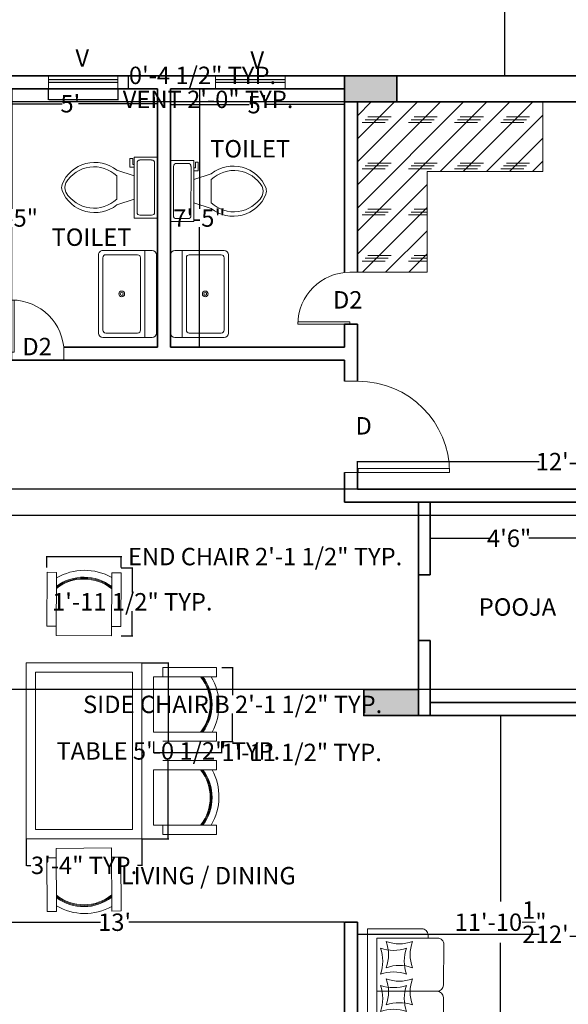
# Model space of a CAD drawing. Units: inches. Extents: x -2181 to 1225, y -80 to 4016.
# Tile 3 of 10: x 308 to 497, y 253 to 592. Entities that reach past the tile are written whole.
import ezdxf

# ---------------------------------------------------------------- set-up
doc = ezdxf.new("R2010")
doc.units = ezdxf.units.IN
doc.header["$MEASUREMENT"] = 0
for name, color, linetype, lineweight in [('A-ANNO-DIMS', 2, 'Continuous', 18), ('A-ANNO-TEXT', 7, 'Continuous', 18), ('A-AREA-IDEN', 7, 'Continuous', 18), ('A-COLS', 7, 'Continuous', 35), ('A-COLS-PATT', 252, 'Continuous', 13), ('A-DOOR', 3, 'Continuous', 18), ('A-FLOR-FIXT', 8, 'Continuous', 18), ('A-FURN', 30, 'Continuous', 18), ('A-GLAZ', 4, 'Continuous', 18), ('A-GLAZ-PATT', 4, 'Continuous', 13), ('A-MILL', 8, 'Continuous', 18), ('A-MILL-PATT', 252, 'Continuous', 13), ('A-WALL', 7, 'Continuous', 35)]:
    doc.layers.add(name, color=color, linetype=linetype, lineweight=lineweight)
doc.styles.get("Standard").update_dxf_attribs({"font": 'arial.ttf'})
doc.dimstyles.get("Standard").update_dxf_attribs({"dimtxt": 6, "dimasz": 0.18, "dimexe": 0.18, "dimexo": 0.0625, "dimgap": 0.09, "dimtad": 0, "dimtih": 1, "dimtoh": 1, "dimdec": 4, "dimzin": 0, "dimdsep": 46, "dimlunit": 4, "dimtxsty": 'Standard', "dimcen": 0.09, "dimadec": 0, "dimazin": 0, "dimtfac": 1, "dimtdec": 4, "dimtofl": 0, "dimtmove": 0, "dimatfit": 3, "dimfxl": 1, "dimtolj": 1, "dimtzin": 0, "dimarcsym": 0})

# ---------------------------------------------------------------- blocks, each defined once
blk = doc.blocks.new('*U2')
for p, q in [((0, 0), (0, -6)), ((40, 0), (40, -6))]:
    blk.add_line(p, q)
blk.add_lwpolyline([(0, 0), (0, 40), (1.75, 40), (1.75, 0)], close=True)
blk.add_arc((0, 0), 40, 0, 90)
blk = doc.blocks.new('*U21')
for p, q in [((9.5, -6), (9.5, -2)), ((-10, -8.5), (-8, -8.5)), ((-10, -9.5), (-10, -8.5)), ((-7, -9.5), (-10, -9.5)), ((-8, -8.5), (-8, -8)), ((-7, -8), (-7, -9.5)), ((-4, -8), (-6, -14)), ((4, -8), (6, -14)), ((4, -14), (-4, -14))]:
    blk.add_line(p, q)
blk.add_lwpolyline([(10.5, -8), (10.5, 0), (-10.5, 0), (-10.5, -8)], close=True)
for points in [[(-9.5, -2), (-9.5, -6)], [(8.5, -1), (-8.5, -1)], [(-8.5, -7), (8.5, -7)]]:
    blk.add_lwpolyline(points)
for centre, radius, start, end in [((-8.62, -1.88), 0.884, 81.8699, 188.1301), ((8.62, -1.88), 0.884, 351.8699, 98.1301), ((-8.62, -6.12), 0.884, 171.8699, 278.1301), ((8.62, -6.12), 0.884, 261.8699, 8.1301), ((3.52, -21.58), 12.17, 141.4691, 247.9714), ((4.2, -21.82), 11.33, 136.3677, 238.9468), ((-3.52, -21.58), 12.17, 292.0284, 38.5307), ((-4.2, -21.82), 11.33, 301.053, 43.6321), ((0, -27.88), 4, 245.7318, 294.2682), ((0, -29), 4, 254.8605, 285.1395)]:
    blk.add_arc(centre, radius, start, end)
blk = doc.blocks.new('Sink-single - 30 in top')
blk.add_line((-15, -3.999996), (15, -3.999996))
for points in [[(-13.5, 0), (13.5, 0)], [(-15, -18.499996), (-15, -1.5)], [(15, -1.5), (15, -18.499996)], [(-13.5, -17.499996), (-13.5, -6.499996)], [(-12.5, -5.499996), (12.5, -5.499996)], [(13.5, -6.499996), (13.5, -17.499996)], [(13.5, -19.999996), (-13.5, -19.999996)], [(12.5, -18.499996), (-12.5, -18.499996)]]:
    blk.add_lwpolyline(points)
for radius in [1, 0.5]:
    blk.add_circle((0, -11.999996), radius)
for centre, radius, start, end in [((-13.5, -1.5), 1.5, 90, 180), ((13.5, -1.5), 1.5, 0, 90), ((-12.5, -6.499996), 1, 90, 180), ((12.5, -6.499996), 1, 0, 90), ((-13.5, -18.499996), 1.5, 180, 270), ((-12.5, -17.499996), 1, 180, 270), ((12.5, -17.499996), 1, 270, 0), ((13.5, -18.499996), 1.5, 270, 0)]:
    blk.add_arc(centre, radius, start, end)
blk = doc.blocks.new('*D22')
at = {"layer": 'A-ANNO-DIMS', "color": 0, "lineweight": -2, "transparency": 16777216}
for p, q in [((470.02, 664.48), (474.9, 664.48)), ((474.72, 664.3), (474.72, 625.85)), ((474.72, 573.16), (474.72, 611.62)), ((624.01, 572.98), (474.54, 572.98))]:
    blk.add_line(p, q, dxfattribs=at)
at = {"layer": 'A-ANNO-DIMS', "color": 0, "transparency": 16777216}
for points in [[(474.69, 664.3), (474.75, 664.3), (474.72, 664.48)], [(474.69, 573.16), (474.75, 573.16), (474.72, 572.98)]]:
    blk.add_solid(points, dxfattribs=at)
at = {"layer": 'Defpoints', "color": 0, "transparency": 16777216}
for p in [(469.95, 664.48), (474.72, 572.98), (624.08, 572.98)]:
    blk.add_point(p, dxfattribs=at)
at = {"layer": 'A-ANNO-DIMS', "color": 0, "transparency": 16777216, "insert": (474.72, 618.73), "char_height": 6, "attachment_point": 5}
blk.add_mtext('\\A1;7\'-7{\\H1x;\\S1/2;}"', dxfattribs=at)
blk = doc.blocks.new('*D26')
at = {"layer": 'A-ANNO-DIMS', "color": 0, "lineweight": -2, "transparency": 16777216}
for p, q in [((295.08, 568.48), (305, 568.48)), ((304.82, 568.3), (304.82, 527.13)), ((304.82, 479.66), (304.82, 520.84)), ((295.08, 479.48), (305, 479.48))]:
    blk.add_line(p, q, dxfattribs=at)
at = {"layer": 'A-ANNO-DIMS', "color": 0, "transparency": 16777216}
for points in [[(304.79, 568.3), (304.85, 568.3), (304.82, 568.48)], [(304.79, 479.66), (304.85, 479.66), (304.82, 479.48)]]:
    blk.add_solid(points, dxfattribs=at)
at = {"layer": 'Defpoints', "color": 0, "transparency": 16777216}
for p in [(295.01, 568.48), (295.01, 479.48), (304.82, 479.48)]:
    blk.add_point(p, dxfattribs=at)
at = {"layer": 'A-ANNO-DIMS', "color": 0, "transparency": 16777216, "insert": (304.82, 523.98), "char_height": 6, "attachment_point": 5}
blk.add_mtext('\\A1;7\'-5"', dxfattribs=at)
blk = doc.blocks.new('*D27')
at = {"layer": 'A-ANNO-DIMS', "color": 0, "lineweight": -2, "transparency": 16777216}
for p, q in [((359.58, 568.48), (369.69, 568.48)), ((369.51, 568.3), (369.51, 527.13)), ((369.51, 479.66), (369.51, 520.84)), ((359.58, 479.48), (369.69, 479.48))]:
    blk.add_line(p, q, dxfattribs=at)
at = {"layer": 'A-ANNO-DIMS', "color": 0, "transparency": 16777216}
for points in [[(369.48, 568.3), (369.54, 568.3), (369.51, 568.48)], [(369.48, 479.66), (369.54, 479.66), (369.51, 479.48)]]:
    blk.add_solid(points, dxfattribs=at)
at = {"layer": 'Defpoints', "color": 0, "transparency": 16777216}
for p in [(359.51, 568.48), (359.51, 479.48), (369.51, 479.48)]:
    blk.add_point(p, dxfattribs=at)
at = {"layer": 'A-ANNO-DIMS', "color": 0, "transparency": 16777216, "insert": (369.51, 523.98), "char_height": 6, "attachment_point": 5}
blk.add_mtext('\\A1;7\'-5"', dxfattribs=at)
blk = doc.blocks.new('*D28')
at = {"layer": 'A-ANNO-DIMS', "color": 0, "lineweight": -2, "transparency": 16777216}
for p, q in [((295.01, 568.42), (295.01, 563.2)), ((355.01, 568.42), (355.01, 563.2)), ((295.19, 563.38), (322.16, 563.38)), ((354.83, 563.38), (327.87, 563.38))]:
    blk.add_line(p, q, dxfattribs=at)
at = {"layer": 'A-ANNO-DIMS', "color": 0, "transparency": 16777216}
for points in [[(295.19, 563.41), (295.19, 563.35), (295.01, 563.38)], [(354.83, 563.41), (354.83, 563.35), (355.01, 563.38)]]:
    blk.add_solid(points, dxfattribs=at)
at = {"layer": 'Defpoints', "color": 0, "transparency": 16777216}
for p in [(295.01, 568.48), (355.01, 568.48), (355.01, 563.38)]:
    blk.add_point(p, dxfattribs=at)
at = {"layer": 'A-ANNO-DIMS', "color": 0, "transparency": 16777216, "insert": (325.01, 563.38), "char_height": 6, "attachment_point": 5}
blk.add_mtext("\\A1;5'", dxfattribs=at)
blk = doc.blocks.new('*D29')
at = {"layer": 'A-ANNO-DIMS', "color": 0, "lineweight": -2, "transparency": 16777216}
for p, q in [((359.51, 568.42), (359.51, 562.88)), ((419.51, 568.42), (419.51, 562.88)), ((359.69, 563.06), (386.66, 563.06)), ((419.33, 563.06), (392.37, 563.06))]:
    blk.add_line(p, q, dxfattribs=at)
at = {"layer": 'A-ANNO-DIMS', "color": 0, "transparency": 16777216}
for points in [[(359.69, 563.09), (359.69, 563.03), (359.51, 563.06)], [(419.33, 563.09), (419.33, 563.03), (419.51, 563.06)]]:
    blk.add_solid(points, dxfattribs=at)
at = {"layer": 'Defpoints', "color": 0, "transparency": 16777216}
for p in [(359.51, 568.48), (419.51, 568.48), (419.51, 563.06)]:
    blk.add_point(p, dxfattribs=at)
at = {"layer": 'A-ANNO-DIMS', "color": 0, "transparency": 16777216, "insert": (389.51, 563.06), "char_height": 6, "attachment_point": 5}
blk.add_mtext("\\A1;5'", dxfattribs=at)
blk = doc.blocks.new('*D43')
at = {"layer": 'A-ANNO-DIMS', "color": 0, "lineweight": -2, "transparency": 16777216}
for p, q in [((424.01, 281.17), (424.01, 276.89)), ((424.19, 277.07), (486.63, 277.07)), ((578.33, 277.07), (515.9, 277.07)), ((578.51, 277.13), (578.51, 277.25))]:
    blk.add_line(p, q, dxfattribs=at)
at = {"layer": 'A-ANNO-DIMS', "color": 0, "transparency": 16777216}
for points in [[(424.19, 277.1), (424.19, 277.04), (424.01, 277.07)], [(578.33, 277.1), (578.33, 277.04), (578.51, 277.07)]]:
    blk.add_solid(points, dxfattribs=at)
at = {"layer": 'Defpoints', "color": 0, "transparency": 16777216}
for p in [(424.01, 281.23), (578.51, 277.07), (578.51, 277.07)]:
    blk.add_point(p, dxfattribs=at)
at = {"layer": 'A-ANNO-DIMS', "color": 0, "transparency": 16777216, "insert": (501.26, 277.07), "char_height": 6, "attachment_point": 5}
blk.add_mtext('\\A1;12\'-10{\\H1x;\\S1/2;}"', dxfattribs=at)
blk = doc.blocks.new('*D44')
at = {"layer": 'A-ANNO-DIMS', "color": 0, "lineweight": -2, "transparency": 16777216}
for p, q in [((473.3, 352.3), (473.3, 288.4)), ((473.37, 352.48), (473.48, 352.48)), ((473.3, 210.16), (473.3, 274.07)), ((473.37, 209.98), (473.48, 209.98))]:
    blk.add_line(p, q, dxfattribs=at)
at = {"layer": 'A-ANNO-DIMS', "color": 0, "transparency": 16777216}
for points in [[(473.27, 352.3), (473.33, 352.3), (473.3, 352.48)], [(473.27, 210.16), (473.33, 210.16), (473.3, 209.98)]]:
    blk.add_solid(points, dxfattribs=at)
at = {"layer": 'Defpoints', "color": 0, "transparency": 16777216}
for p in [(473.3, 352.48), (473.3, 352.48), (473.3, 209.98)]:
    blk.add_point(p, dxfattribs=at)
at = {"layer": 'A-ANNO-DIMS', "color": 0, "transparency": 16777216, "insert": (473.3, 281.23), "char_height": 6, "attachment_point": 5}
blk.add_mtext('\\A1;11\'-10{\\H1x;\\S1/2;}"', dxfattribs=at)
blk = doc.blocks.new('*D45')
at = {"layer": 'A-ANNO-DIMS', "color": 0, "lineweight": -2, "transparency": 16777216}
for p, q in [((449.01, 425.92), (449.01, 413.4)), ((503.46, 425.92), (503.46, 413.4)), ((449.19, 413.58), (469.45, 413.58)), ((503.28, 413.58), (483.03, 413.58))]:
    blk.add_line(p, q, dxfattribs=at)
at = {"layer": 'A-ANNO-DIMS', "color": 0, "transparency": 16777216}
for points in [[(449.19, 413.61), (449.19, 413.55), (449.01, 413.58)], [(503.28, 413.61), (503.28, 413.55), (503.46, 413.58)]]:
    blk.add_solid(points, dxfattribs=at)
at = {"layer": 'Defpoints', "color": 0, "transparency": 16777216}
for p in [(449.01, 425.98), (503.46, 425.98), (503.46, 413.58)]:
    blk.add_point(p, dxfattribs=at)
at = {"layer": 'A-ANNO-DIMS', "color": 0, "transparency": 16777216, "insert": (476.24, 413.58), "char_height": 6, "width": 24.618, "attachment_point": 5}
blk.add_mtext('\\A1;4\'6"', dxfattribs=at)
blk = doc.blocks.new('*D48')
at = {"layer": 'A-ANNO-DIMS', "color": 0, "lineweight": -2, "transparency": 16777216}
for p, q in [((424.01, 430.55), (424.01, 440.19)), ((424.19, 440.01), (486.63, 440.01)), ((578.33, 440.01), (515.9, 440.01)), ((578.51, 430.55), (578.51, 440.19))]:
    blk.add_line(p, q, dxfattribs=at)
at = {"layer": 'A-ANNO-DIMS', "color": 0, "transparency": 16777216}
for points in [[(424.19, 440.04), (424.19, 439.98), (424.01, 440.01)], [(578.33, 440.04), (578.33, 439.98), (578.51, 440.01)]]:
    blk.add_solid(points, dxfattribs=at)
at = {"layer": 'Defpoints', "color": 0, "transparency": 16777216}
for p in [(578.51, 440.01), (424.01, 430.48), (578.51, 430.48)]:
    blk.add_point(p, dxfattribs=at)
at = {"layer": 'A-ANNO-DIMS', "color": 0, "transparency": 16777216, "insert": (501.26, 440.01), "char_height": 6, "attachment_point": 5}
blk.add_mtext('\\A1;12\'-10{\\H1x;\\S1/2;}"', dxfattribs=at)
blk = doc.blocks.new('*D49')
at = {"layer": 'A-ANNO-DIMS', "color": 0, "lineweight": -2, "transparency": 16777216}
for p, q in [((261.01, 284.15), (261.01, 281.05)), ((261.19, 281.23), (335.37, 281.23)), ((419.33, 281.23), (345.16, 281.23)), ((419.51, 281.3), (419.51, 281.41))]:
    blk.add_line(p, q, dxfattribs=at)
at = {"layer": 'A-ANNO-DIMS', "color": 0, "transparency": 16777216}
for points in [[(261.19, 281.26), (261.19, 281.2), (261.01, 281.23)], [(419.33, 281.26), (419.33, 281.2), (419.51, 281.23)]]:
    blk.add_solid(points, dxfattribs=at)
at = {"layer": 'Defpoints', "color": 0, "transparency": 16777216}
for p in [(261.01, 284.21), (419.51, 281.23), (419.51, 281.23)]:
    blk.add_point(p, dxfattribs=at)
at = {"layer": 'A-ANNO-DIMS', "color": 0, "transparency": 16777216, "insert": (340.26, 281.23), "char_height": 6, "attachment_point": 5}
blk.add_mtext("\\A1;13'", dxfattribs=at)
blk = doc.blocks.new('*D71')
at = {"layer": 'A-ANNO-DIMS', "color": 0, "lineweight": -2, "transparency": 16777216}
for p, q in [((98.51, 573.05), (98.51, 611.58)), ((98.69, 611.4), (536.64, 611.4)), ((995.33, 611.4), (557.39, 611.4)), ((995.51, 573.05), (995.51, 611.58))]:
    blk.add_line(p, q, dxfattribs=at)
at = {"layer": 'A-ANNO-DIMS', "color": 0, "transparency": 16777216}
for points in [[(98.69, 611.43), (98.69, 611.37), (98.51, 611.4)], [(995.33, 611.43), (995.33, 611.37), (995.51, 611.4)]]:
    blk.add_solid(points, dxfattribs=at)
at = {"layer": 'Defpoints', "color": 0, "transparency": 16777216}
for p in [(995.51, 611.4), (98.51, 572.98), (995.51, 572.98)]:
    blk.add_point(p, dxfattribs=at)
at = {"layer": 'A-ANNO-DIMS', "color": 0, "transparency": 16777216, "insert": (547.01, 611.4), "char_height": 6, "attachment_point": 5}
blk.add_mtext('\\A1;74\'-9"', dxfattribs=at)
blk = doc.blocks.new('SOFA-UPHOLSTERED')
for p, q in [((3.23, 44.91), (24.04, 44.91)), ((3.23, 22.57), (24.04, 22.58)), ((25.11, 22.58), (25.11, 22.58))]:
    blk.add_line(p, q)
for points in [[(0, 0), (0, 66.42), (18.76, 66.42, -0.414214), (20.91, 64.27), (20.91, 63.19)], [(3.23, 3.23), (3.23, 63.19), (24.21, 63.19, -0.417877), (26.36, 61.02), (26.19, 47.04, -0.410559), (24.04, 44.91), (3.23, 44.91)], [(26.19, 42.76), (26.19, 24.73, -0.414214), (24.04, 22.58), (3.23, 22.58)], [(26.19, 20.43), (26.19, 5.38, -0.414214), (24.04, 3.23), (3.23, 3.23)], [(21.99, 3.23), (21.99, 3.23, -0.414214), (18.76, 0), (0, 0)]]:
    blk.add_lwpolyline(points, format="xyb")
for points in [[(18.76, 66.42), (19, 66.42)], [(19, 0), (18.76, 0)]]:
    blk.add_lwpolyline(points)
for centre, radius, start, end in [((11.03, 74.56), 13.33, 250.2663, 289.7337), ((-6.02, 57.51), 13.33, 340.2663, 19.7337), ((28.07, 57.51), 13.33, 160.2663, 199.7337), ((9.03, 72.31), 13.33, 250.2663, 289.7337), ((-8.02, 55.27), 13.33, 340.2663, 19.7337), ((26.07, 55.27), 13.33, 160.2663, 199.7337), ((9.03, 38.22), 13.33, 70.2663, 109.7337), ((11.03, 40.47), 13.33, 70.2663, 109.7337), ((11.03, 61.71), 13.33, 250.2663, 289.7337), ((-6.02, 44.66), 13.33, 340.2663, 19.7337), ((28.07, 44.66), 13.33, 160.2663, 199.7337), ((9.03, 59.47), 13.33, 250.2663, 289.7337), ((-8.02, 42.42), 13.33, 340.2663, 19.7337), ((26.07, 42.42), 13.33, 160.2663, 199.7337), ((24.04, 42.76), 2.15, 360, 90), ((11.03, 27.62), 13.33, 70.2663, 109.7337), ((9.03, 25.38), 13.33, 70.2663, 109.7337), ((11.72, 48.03), 13.33, 250.2663, 289.7337), ((-5.33, 30.99), 13.33, 340.2663, 19.7337), ((28.76, 30.99), 13.33, 160.2663, 199.7337), ((9.72, 45.79), 13.33, 250.2663, 289.7337), ((-7.33, 28.74), 13.33, 340.2663, 19.7337), ((26.76, 28.74), 13.33, 160.2663, 199.7337), ((11.72, 13.94), 13.33, 70.2663, 109.7337), ((9.72, 11.7), 13.33, 70.2663, 109.7337), ((24.04, 20.43), 2.15, 0, 90.0249), ((9.86, 27), 13.33, 250.2663, 289.7337), ((-7.19, 9.96), 13.33, 340.2663, 19.7337), ((11.86, 29.25), 13.33, 250.2663, 289.7337), ((-5.19, 12.2), 13.33, 340.2663, 19.7337), ((26.9, 9.96), 13.33, 160.2663, 199.7337), ((28.9, 12.2), 13.33, 160.2663, 199.7337), ((11.86, -4.84), 13.33, 70.2663, 109.7337), ((9.86, -7.09), 13.33, 70.2663, 109.7337)]:
    blk.add_arc(centre, radius, start, end)
blk = doc.blocks.new('DINING-CHAIR-SIDE-B')
for p, q in [((3.21, 22.26), (3.21, 25.47)), ((21.75, 22.26), (21.75, 25.47)), ((21.75, 0), (21.75, 3.21))]:
    blk.add_line(p, q)
for points in [[(21.75, 25.47), (3.21, 25.47)], [(21.75, 22.26), (0, 22.26), (0, 3.21), (21.75, 3.21)], [(3.21, 0), (21.75, 0)]]:
    blk.add_lwpolyline(points)
for centre, radius, start, end in [((4.25, 12.73), 15.28, 321.4242, 38.5758), ((4.25, 12.73), 15.6, 322.3578, 37.6422), ((4.25, 12.73), 15.92, 323.2428, 36.7572), ((3.41, 12.45), 19.13, 331.1027, 30.8582)]:
    blk.add_arc(centre, radius, start, end)
blk = doc.blocks.new('DINING-CHAIR-END')
for p, q in [((3.21, 19.25), (0, 19.23)), ((22.26, 19.4), (25.47, 19.42)), ((25.38, 19.42), (25.38, 19.34)), ((3.35, 0.72), (0.14, 0.69)), ((25.61, 0.89), (22.4, 0.86))]:
    blk.add_line(p, q)
for points in [[(3.35, 0.72), (3.18, 22.46), (22.23, 22.61), (22.4, 0.86)], [(0.14, 0.69), (0, 19.23)], [(25.47, 19.42), (25.61, 0.89)]]:
    blk.add_lwpolyline(points)
for centre, radius, start, end in [((12.74, 18.29), 15.28, 231.8612, 309.0129), ((12.74, 18.29), 15.6, 232.7948, 308.0793), ((12.74, 18.29), 15.92, 233.6799, 307.1942), ((13.02, 19.13), 19.13, 239.5789, 299.3344)]:
    blk.add_arc(centre, radius, start, end)
blk = doc.blocks.new('DINING-TABLE')
for points in [[(39.83, 60.67), (39.83, 0), (0, 0), (0, 60.67)], [(36.62, 57.46), (36.62, 3.21), (3.21, 3.21), (3.21, 57.46)]]:
    blk.add_lwpolyline(points, close=True)
blk = doc.blocks.new('COL-18X9')
blk.add_lwpolyline([(0, 9), (18, 9), (18, 0), (0, 0)], close=True)
blk = doc.blocks.new('COL-18.89X9')
blk.add_lwpolyline([(18.9, 9), (0, 9), (0, 0), (18.9, 0)], close=True)
blk = doc.blocks.new('VENT-24')
for p, q in [((0, 0), (0, 4.5)), ((24, 0), (24, 4.5)), ((0, 3.25), (24, 3.25)), ((0, 2.25), (24, 2.25))]:
    blk.add_line(p, q)
blk = doc.blocks.new('*D100')
at = {"layer": 'A-ANNO-DIMS', "color": 0, "lineweight": -2, "transparency": 16777216}
for p, q in [((316.92, 403.49), (316.92, 407.45)), ((342.53, 403.49), (342.53, 407.45)), ((317.1, 407.27), (342.35, 407.27)), ((342.53, 407.27), (342.71, 407.27))]:
    blk.add_line(p, q, dxfattribs=at)
at = {"layer": 'A-ANNO-DIMS', "color": 0, "transparency": 16777216}
for points in [[(317.1, 407.3), (317.1, 407.24), (316.92, 407.27)], [(342.35, 407.3), (342.35, 407.24), (342.53, 407.27)]]:
    blk.add_solid(points, dxfattribs=at)
at = {"layer": 'Defpoints', "color": 0, "transparency": 16777216}
for p in [(342.53, 407.27), (316.92, 403.43), (342.53, 403.43)]:
    blk.add_point(p, dxfattribs=at)
at = {"layer": 'A-ANNO-DIMS', "color": 0, "transparency": 16777216, "insert": (392.14, 407.27), "char_height": 6, "attachment_point": 5}
blk.add_mtext('\\A1;END CHAIR 2\'-1 1/2" TYP.', dxfattribs=at)
blk = doc.blocks.new('*D101')
at = {"layer": 'A-ANNO-DIMS', "color": 0, "lineweight": -2, "transparency": 16777216}
for p, q in [((342.59, 403.43), (346.55, 403.43)), ((346.37, 403.25), (346.37, 394.87)), ((346.37, 380.12), (346.37, 388.49)), ((342.59, 379.94), (346.55, 379.94))]:
    blk.add_line(p, q, dxfattribs=at)
at = {"layer": 'A-ANNO-DIMS', "color": 0, "transparency": 16777216}
for points in [[(346.34, 403.25), (346.4, 403.25), (346.37, 403.43)], [(346.34, 380.12), (346.4, 380.12), (346.37, 379.94)]]:
    blk.add_solid(points, dxfattribs=at)
at = {"layer": 'Defpoints', "color": 0, "transparency": 16777216}
for p in [(342.53, 403.43), (342.53, 379.94), (346.37, 379.94)]:
    blk.add_point(p, dxfattribs=at)
at = {"layer": 'A-ANNO-DIMS', "color": 0, "transparency": 16777216, "insert": (346.37, 391.68), "char_height": 6, "attachment_point": 5}
blk.add_mtext('\\A1;1\'-11 1/2" TYP.', dxfattribs=at)
blk = doc.blocks.new('*D108')
at = {"layer": 'A-ANNO-DIMS', "color": 0, "lineweight": -2, "transparency": 16777216}
for p, q in [((377.2, 369.05), (381.14, 369.05)), ((380.96, 368.87), (380.96, 359.51)), ((380.96, 343.76), (380.96, 353.12)), ((377.2, 343.58), (381.14, 343.58))]:
    blk.add_line(p, q, dxfattribs=at)
at = {"layer": 'A-ANNO-DIMS', "color": 0, "transparency": 16777216}
for points in [[(380.93, 368.87), (380.99, 368.87), (380.96, 369.05)], [(380.93, 343.76), (380.99, 343.76), (380.96, 343.58)]]:
    blk.add_solid(points, dxfattribs=at)
at = {"layer": 'Defpoints', "color": 0, "transparency": 16777216}
for p in [(377.14, 369.05), (380.96, 369.05), (377.14, 343.58)]:
    blk.add_point(p, dxfattribs=at)
at = {"layer": 'A-ANNO-DIMS', "color": 0, "transparency": 16777216, "insert": (380.96, 356.32), "char_height": 6, "attachment_point": 5}
blk.add_mtext('\\A1;SIDE CHAIR B 2\'-1 1/2" TYP.', dxfattribs=at)
blk = doc.blocks.new('*D109')
at = {"layer": 'A-ANNO-DIMS', "color": 0, "lineweight": -2, "transparency": 16777216}
for p, q in [((353.7, 343.52), (353.7, 339.58)), ((377.14, 343.52), (377.14, 339.58)), ((353.88, 339.76), (376.96, 339.76)), ((377.14, 339.76), (377.32, 339.76))]:
    blk.add_line(p, q, dxfattribs=at)
at = {"layer": 'A-ANNO-DIMS', "color": 0, "transparency": 16777216}
for points in [[(353.88, 339.79), (353.88, 339.73), (353.7, 339.76)], [(376.96, 339.79), (376.96, 339.73), (377.14, 339.76)]]:
    blk.add_solid(points, dxfattribs=at)
at = {"layer": 'Defpoints', "color": 0, "transparency": 16777216}
for p in [(353.7, 343.58), (377.14, 343.58), (377.14, 339.76)]:
    blk.add_point(p, dxfattribs=at)
at = {"layer": 'A-ANNO-DIMS', "color": 0, "transparency": 16777216, "insert": (404.73, 339.76), "char_height": 6, "attachment_point": 5}
blk.add_mtext('\\A1;1\'-11 1/2" TYP.', dxfattribs=at)
blk = doc.blocks.new('*D110')
at = {"layer": 'A-ANNO-DIMS', "color": 0, "lineweight": -2, "transparency": 16777216}
for p, q in [((349.74, 370.6), (358.96, 370.6)), ((358.78, 370.42), (358.78, 343.46)), ((358.78, 310.11), (358.78, 337.07)), ((349.74, 309.93), (358.96, 309.93))]:
    blk.add_line(p, q, dxfattribs=at)
at = {"layer": 'A-ANNO-DIMS', "color": 0, "transparency": 16777216}
for points in [[(358.75, 370.42), (358.81, 370.42), (358.78, 370.6)], [(358.75, 310.11), (358.81, 310.11), (358.78, 309.93)]]:
    blk.add_solid(points, dxfattribs=at)
at = {"layer": 'Defpoints', "color": 0, "transparency": 16777216}
for p in [(349.68, 370.6), (358.78, 370.6), (349.68, 309.93)]:
    blk.add_point(p, dxfattribs=at)
at = {"layer": 'A-ANNO-DIMS', "color": 0, "transparency": 16777216, "insert": (358.78, 340.27), "char_height": 6, "attachment_point": 5}
blk.add_mtext('\\A1;TABLE 5\'-0 1/2" TYP.', dxfattribs=at)
blk = doc.blocks.new('*D111')
at = {"layer": 'A-ANNO-DIMS', "color": 0, "lineweight": -2, "transparency": 16777216}
for p, q in [((309.85, 309.87), (309.85, 300.65)), ((349.68, 309.87), (349.68, 300.65)), ((310.03, 300.83), (311.39, 300.83)), ((349.5, 300.83), (348.14, 300.83))]:
    blk.add_line(p, q, dxfattribs=at)
at = {"layer": 'A-ANNO-DIMS', "color": 0, "transparency": 16777216}
for points in [[(310.03, 300.86), (310.03, 300.8), (309.85, 300.83)], [(349.5, 300.86), (349.5, 300.8), (349.68, 300.83)]]:
    blk.add_solid(points, dxfattribs=at)
at = {"layer": 'Defpoints', "color": 0, "transparency": 16777216}
for p in [(309.85, 309.93), (349.68, 309.93), (349.68, 300.83)]:
    blk.add_point(p, dxfattribs=at)
at = {"layer": 'A-ANNO-DIMS', "color": 0, "transparency": 16777216, "insert": (329.76, 300.83), "char_height": 6, "attachment_point": 5}
blk.add_mtext('\\A1;3\'-4" TYP.', dxfattribs=at)
blk = doc.blocks.new('*D126')
at = {"layer": 'A-ANNO-DIMS', "color": 0, "lineweight": -2, "transparency": 16777216}
for p, q in [((317.43, 568.42), (317.43, 564.7)), ((341.43, 568.42), (341.43, 564.7)), ((317.61, 564.88), (341.25, 564.88)), ((341.43, 564.88), (341.61, 564.88))]:
    blk.add_line(p, q, dxfattribs=at)
at = {"layer": 'A-ANNO-DIMS', "color": 0, "transparency": 16777216}
for points in [[(317.61, 564.91), (317.61, 564.85), (317.43, 564.88)], [(341.25, 564.91), (341.25, 564.85), (341.43, 564.88)]]:
    blk.add_solid(points, dxfattribs=at)
at = {"layer": 'Defpoints', "color": 0, "transparency": 16777216}
for p in [(317.43, 568.48), (341.43, 568.48), (341.43, 564.88)]:
    blk.add_point(p, dxfattribs=at)
at = {"layer": 'A-ANNO-DIMS', "color": 0, "transparency": 16777216, "insert": (372.49, 564.88), "char_height": 6, "attachment_point": 5}
blk.add_mtext('\\A1;VENT 2\'-0" TYP.', dxfattribs=at)
blk = doc.blocks.new('*D127')
at = {"layer": 'A-ANNO-DIMS', "color": 0, "lineweight": -2, "transparency": 16777216}
for p, q in [((341.5, 572.98), (345.21, 572.98)), ((345.03, 572.98), (345.03, 573.16)), ((345.03, 573.16), (345.21, 573.16)), ((345.03, 568.66), (345.03, 572.8)), ((341.5, 568.48), (345.21, 568.48))]:
    blk.add_line(p, q, dxfattribs=at)
at = {"layer": 'A-ANNO-DIMS', "color": 0, "transparency": 16777216}
for points in [[(345, 572.8), (345.06, 572.8), (345.03, 572.98)], [(345, 568.66), (345.06, 568.66), (345.03, 568.48)]]:
    blk.add_solid(points, dxfattribs=at)
at = {"layer": 'Defpoints', "color": 0, "transparency": 16777216}
for p in [(341.43, 572.98), (345.03, 572.98), (341.43, 568.48)]:
    blk.add_point(p, dxfattribs=at)
at = {"layer": 'A-ANNO-DIMS', "color": 0, "transparency": 16777216, "insert": (370.58, 573.16), "char_height": 6, "attachment_point": 5}
blk.add_mtext('\\A1;0\'-4 1/2" TYP.', dxfattribs=at)
blk = doc.blocks.new('*D130')
at = {"layer": 'A-ANNO-DIMS', "color": 0, "lineweight": -2, "transparency": 16777216}
for p, q in [((512.45, 421.48), (-59.44, 421.48)), ((-59.26, 421.3), (-59.26, 394.64)), ((-59.26, 361.66), (-59.26, 388.33)), ((512.45, 361.48), (-59.44, 361.48))]:
    blk.add_line(p, q, dxfattribs=at)
at = {"layer": 'A-ANNO-DIMS', "color": 0, "transparency": 16777216}
for points in [[(-59.29, 421.3), (-59.23, 421.3), (-59.26, 421.48)], [(-59.29, 361.66), (-59.23, 361.66), (-59.26, 361.48)]]:
    blk.add_solid(points, dxfattribs=at)
at = {"layer": 'Defpoints', "color": 0, "transparency": 16777216}
for p in [(512.51, 421.48), (-59.26, 361.48), (512.51, 361.48)]:
    blk.add_point(p, dxfattribs=at)
at = {"layer": 'A-ANNO-DIMS', "color": 0, "transparency": 16777216, "insert": (-59.26, 391.48), "char_height": 6, "attachment_point": 5}
blk.add_mtext('\\A1;5\'-0"', dxfattribs=at)
blk = doc.blocks.new('*D131')
at = {"layer": 'A-ANNO-DIMS', "color": 0, "lineweight": -2, "transparency": 16777216}
for p, q in [((976.64, 563.98), (-59.44, 563.98)), ((-59.26, 563.8), (-59.26, 500.43)), ((-59.26, 430.66), (-59.26, 494.04)), ((977.45, 430.48), (-59.44, 430.48))]:
    blk.add_line(p, q, dxfattribs=at)
at = {"layer": 'A-ANNO-DIMS', "color": 0, "transparency": 16777216}
for points in [[(-59.29, 563.8), (-59.23, 563.8), (-59.26, 563.98)], [(-59.29, 430.66), (-59.23, 430.66), (-59.26, 430.48)]]:
    blk.add_solid(points, dxfattribs=at)
at = {"layer": 'Defpoints', "color": 0, "transparency": 16777216}
for p in [(976.7, 563.98), (-59.26, 430.48), (977.51, 430.48)]:
    blk.add_point(p, dxfattribs=at)
at = {"layer": 'A-ANNO-DIMS', "color": 0, "transparency": 16777216, "insert": (-59.26, 497.23), "char_height": 6, "attachment_point": 5}
blk.add_mtext('\\A1;11\'-1 1/2"', dxfattribs=at)

msp = doc.modelspace()

# ---------------------------------------------------------------- hatches: boundary and pattern name
at = {"layer": 'A-COLS-PATT'}
h = msp.add_hatch(color=256, dxfattribs=at)
h.dxf.hatch_style = 1
h.paths.add_polyline_path([(437.51461, 572.98479), (419.51461, 572.98479), (419.51461, 563.98479), (437.51461, 563.98479)])
h.paths.add_polyline_path([(269.65161, 572.98479), (251.65161, 572.98479), (251.65161, 563.98479), (269.65161, 563.98479)])
h.paths.add_polyline_path([(121.82546, 572.98479), (103.01461, 572.98479), (98.51461, 572.98479), (98.51461, 563.98479), (116.51461, 563.98479), (121.82546, 563.98479)])
h.paths.add_polyline_path([(116.51461, 377.48479), (98.51461, 377.48479), (98.51461, 368.48479), (116.51461, 368.48479)])
h.paths.add_polyline_path([(261.01461, 377.48479), (243.01461, 377.48479), (243.01461, 368.48479), (261.01461, 368.48479)])
h = msp.add_hatch(color=256, dxfattribs=at)
h.dxf.hatch_style = 1
h.paths.add_polyline_path([(269.21166, 145.48479), (269.21166, 136.48479), (297.04101, 136.48479), (297.04101, 145.48479)])
h.paths.add_polyline_path([(445.01461, 352.48479), (445.01461, 361.48479), (426.1199, 361.48479), (426.1199, 352.48479)])
h.paths.add_polyline_path([(587.51461, 352.48479), (587.51461, 361.48479), (568.6199, 361.48479), (568.6199, 352.48479)])
h.paths.add_polyline_path([(518.40498, 421.48479), (518.40498, 430.48479), (503.51461, 430.48479), (503.51461, 421.48479)])
h.paths.add_polyline_path([(587.51461, 421.48479), (587.51461, 430.48479), (572.5711, 430.48479), (572.5711, 421.48479)])
at = {"layer": 'A-GLAZ-PATT'}
h = msp.add_hatch(color=256, dxfattribs=at)
h.dxf.hatch_style = 1
h.paths.add_polyline_path([(100.76461, 411.89133), (99.76461, 411.89133), (99.76461, 386.51661), (100.76461, 386.51661)])
h.paths.add_polyline_path([(341.43431, 571.73479), (317.43431, 571.73479), (317.43431, 570.73479), (341.43431, 570.73479)])
h.paths.add_polyline_path([(399.07838, 571.73479), (375.07838, 571.73479), (375.07838, 570.73479), (399.07838, 570.73479)])
at = {"layer": 'A-MILL-PATT'}
h = msp.add_hatch(dxfattribs=at)
h.set_pattern_fill('CORK', color=256, scale=45, angle=45)
h.set_pattern_definition([(45, (0, 0), (-3.977476, 3.977476), []), (180, (3.977, 0), (-2e-15, -15.9099), [7.95495, -7.95495]), (180, (4.972, 0.994), (-2e-15, -15.9099), [7.95495, -7.95495]), (180, (5.966, 1.989), (-2e-15, -15.9099), [7.95495, -7.95495])])
h.paths.add_polyline_path([(487.85532, 563.98479), (424.01461, 563.98479), (424.01461, 539.98479), (487.85532, 539.98479)])
h.paths.add_polyline_path([(448.01461, 539.98479), (424.01461, 539.98479), (424.01461, 505.2672), (448.01461, 505.2672)])

# ---------------------------------------------------------------- linework, layer by layer
at = {"layer": 'A-MILL'}
for p, q in [((487.85532, 539.98479), (487.85532, 563.98479)), ((424.01461, 505.2672), (448.01461, 505.2672))]:
    msp.add_line(p, q, dxfattribs=at)
for points in [[(487.85532, 539.98479), (448.01461, 539.98479)], [(448.01461, 505.2672), (448.01461, 539.98479)]]:
    msp.add_lwpolyline(points, dxfattribs=at)
at = {"layer": 'A-WALL'}
for p, q in [((419.51461, 487.3609), (424.01461, 487.3609)), ((445.01461, 400.99131), (449.01461, 400.99131)), ((445.01461, 378.29291), (449.01461, 378.29291)), ((419.51461, 281.23479), (424.01461, 281.23479))]:
    msp.add_line(p, q, dxfattribs=at)
for points in [[(587.51461, 572.98479), (98.51461, 572.98479), (98.51461, 136.48479)], [(419.51461, 505.17526), (419.51461, 572.98479)], [(355.01461, 568.48479), (295.01461, 568.48479)], [(355.01461, 568.48479), (355.01461, 479.48479)], [(359.51461, 568.48479), (359.51461, 479.48479)], [(419.51461, 568.48479), (359.51461, 568.48479)], [(419.51461, 568.48479), (359.51461, 568.48479)], [(578.51461, 563.98479), (419.51461, 563.98479)], [(578.51461, 563.98479), (424.01461, 563.98479)], [(424.01461, 505.2672), (424.01461, 563.98479)], [(419.51461, 479.48479), (419.51461, 487.3609)], [(424.01461, 467.71596), (424.01461, 487.3609)], [(355.01461, 479.48479), (322.73796, 479.48479)], [(419.51461, 479.48479), (359.51461, 479.48479)], [(359.51461, 474.98479), (295.01461, 474.98479)], [(419.51461, 474.98479), (359.51461, 474.98479)], [(419.51461, 467.71596), (419.51461, 474.98479)], [(419.51461, 425.98479), (419.51461, 436.21069)], [(424.01461, 430.48479), (424.01461, 436.21069)], [(587.51461, 430.48479), (424.01461, 430.48479)], [(449.51461, 425.98479), (419.51461, 425.98479)], [(445.01461, 352.48479), (445.01461, 425.98479)], [(445.01461, 352.48479), (445.01461, 425.98479)], [(449.01461, 400.99131), (449.01461, 425.98479)], [(503.51461, 425.98479), (449.51461, 425.98479)], [(449.01461, 352.48479), (449.01461, 378.29291)], [(503.51461, 356.98479), (449.01461, 356.98479)], [(445.01461, 352.48479), (578.51461, 352.48479)], [(419.51461, 209.98479), (419.51461, 281.23479)], [(424.01461, 209.98479), (424.01461, 281.23479)]]:
    msp.add_lwpolyline(points, dxfattribs=at)

# ---------------------------------------------------------------- block references
at = {"layer": 'A-COLS', "extrusion": (0, 0, -1), "zscale": -1, "rotation": 180}
msp.add_blockref('COL-18X9', (-419.515, 572.98457), dxfattribs=at)
at = {"layer": 'A-COLS'}
msp.add_blockref('COL-18.89X9', (426.11949, 352.485), dxfattribs=at)
at = {"layer": 'A-DOOR'}
for p, xscale, yscale, zscale, rotation in [((421.32735, 487.35209), 0.4478776607911771, 0.4478776607911771, 0.4478776607911771, 90.00000000000003), ((424.2404, 436.21069), -0.7876317507006553, 0.7876317507006553, 0.7876317507006553, 270)]:
    msp.add_blockref('*U2', p, dxfattribs=dict(at, xscale=xscale, yscale=yscale, zscale=zscale, rotation=rotation))
at = {"layer": 'A-DOOR', "xscale": 0.4503069535887608, "yscale": 0.4503069535887608, "zscale": 0.4503069535887608}
msp.add_blockref('*U2', (304.81567, 477.68663), dxfattribs=at)
at = {"layer": 'A-FLOR-FIXT'}
for name, p, rotation in [('*U21', (355.01461, 534.48479), 270), ('Sink-single - 30 in top', (359.51461, 497.80836), 90)]:
    msp.add_blockref(name, p, dxfattribs=dict(at, rotation=rotation))
at = {"layer": 'A-FLOR-FIXT', "xscale": -1}
for name, p, rotation in [('*U21', (359.58885, 533.27976), 89.90827745497215), ('Sink-single - 30 in top', (354.71434, 497.80836), 270)]:
    msp.add_blockref(name, p, dxfattribs=dict(at, rotation=rotation))
at = {"layer": 'A-FURN', "extrusion": (0, 0, -1), "zscale": -1, "rotation": 180}
for name, p in [('DINING-CHAIR-END', (-316.923, 402.54373)), ('DINING-CHAIR-SIDE-B', (-353.695, 336.94878))]:
    msp.add_blockref(name, p, dxfattribs=at)
at = {"layer": 'A-FURN'}
for name, p in [('DINING-TABLE', (309.8467, 309.93185)), ('DINING-CHAIR-SIDE-B', (353.695, 343.583)), ('DINING-CHAIR-END', (316.923, 284.229)), ('SOFA-UPHOLSTERED', (427.379, 212.534))]:
    msp.add_blockref(name, p, dxfattribs=at)
at = {"layer": 'A-GLAZ'}
for p in [(317.434, 568.485), (375.07806, 568.485)]:
    msp.add_blockref('VENT-24', p, dxfattribs=at)

# ---------------------------------------------------------------- texts
at = {"layer": 'A-ANNO-TEXT', "char_height": 6, "attachment_point": 1}
for s, insert in [('V', (326.77133, 582.15216)), ('V', (387.07664, 581.39007)), ('D2', (415.52736, 498.7745)), ('D2', (308.4723, 482.65845)), ('D', (423.29532, 455.34612))]:
    msp.add_mtext_dynamic_manual_height_columns(s, width=291.4178321, gutter_width=1, heights=[0], dxfattribs=dict(at, insert=insert))
at = {"layer": 'A-AREA-IDEN', "char_height": 6, "attachment_point": 1}
for s, heights, insert in [('TOILET', [0], (373.20143, 550.85324)), ('TOILET', [0], (318.55076, 520.37812)), ('POOJA', [6.20873], (465.76675, 392.89157)), ('LIVING / DINING', [0], (342.41525, 300.27334))]:
    msp.add_mtext_dynamic_manual_height_columns(s, width=291.4178321, gutter_width=1, heights=heights, dxfattribs=dict(at, insert=insert))

# ---------------------------------------------------------------- dimensions: what is measured, and where the dimension line sits
at = {"layer": 'A-ANNO-DIMS'}
for base, p1, p2, override, picture, middle in [((474.72038, 572.98479), (469.95283, 664.48479), (624.07639, 572.98479), {"dimclrd": 0, "dimclre": 0, "dimclrt": 0}, '*D22', (474.72038, 618.73479)), ((304.81567, 479.48479), (295.01461, 568.48479), (295.01461, 479.48479), {"dimclrd": 0, "dimclre": 0, "dimclrt": 0}, '*D26', (304.81567, 523.98479)), ((369.51461, 479.48479), (359.51461, 568.48479), (359.51461, 479.48479), {"dimclrd": 0, "dimclre": 0, "dimclrt": 0}, '*D27', (369.51461, 523.98479)), ((-59.2566, 430.48478), (976.70377, 563.98478), (977.51461, 430.48478), {"dimdec": 1, "dimlfac": 1, "dimrnd": 0, "dimzin": 1, "dimdsep": 46, "dimlunit": 4, "dimfrac": 2}, '*D131', (-59.2566, 497.23478)), ((-59.2566, 361.48478), (512.51461, 421.48478), (512.51461, 361.48478), {"dimdec": 1, "dimlfac": 1, "dimrnd": 0, "dimzin": 1, "dimdsep": 46, "dimlunit": 4, "dimfrac": 2}, '*D130', (-59.2566, 391.48478)), ((473.30295, 352.48479), (473.30295, 209.98479), (473.30295, 352.48479), {"dimclrd": 0, "dimclre": 0, "dimclrt": 0}, '*D44', (473.30295, 281.23479))]:
    dim = msp.add_linear_dim(base=base, p1=p1, p2=p2, angle=90, dimstyle='Standard', override=override, dxfattribs=at)
    dim.commit()
    dim.dimension.update_dxf_attribs({"geometry": picture, "text_midpoint": middle})
for base, p1, p2, picture, middle in [((995.51461, 611.40365), (98.51461, 572.98479), (995.51461, 572.98479), '*D71', (547.01461, 611.40365)), ((355.01461, 563.38158), (295.01461, 568.48479), (355.01461, 568.48479), '*D28', (325.01461, 563.38158)), ((419.51461, 563.0638), (359.51461, 568.48479), (419.51461, 568.48479), '*D29', (389.51461, 563.0638)), ((578.51461, 440.00848), (424.01461, 430.48479), (578.51461, 430.48479), '*D48', (501.26461, 440.00848)), ((578.51461, 277.07243), (424.01461, 281.23479), (578.51461, 277.07243), '*D43', (501.26461, 277.07243))]:
    dim = msp.add_linear_dim(base=base, p1=p1, p2=p2, dimstyle='Standard', override={"dimclrd": 0, "dimclre": 0, "dimclrt": 0}, dxfattribs=at)
    dim.commit()
    dim.dimension.update_dxf_attribs({"geometry": picture, "text_midpoint": middle})
for base, p1, p2, angle, text, picture, middle in [((345.03431, 572.98479), (341.43431, 568.48479), (341.43431, 572.98479), 90, '<> TYP.', '*D127', (370.58126, 573.16479)), ((346.37211, 379.9374), (342.53089, 403.4257), (342.53089, 379.9374), 270, '<> TYP.', '*D101', (346.37211, 391.68155)), ((380.95874, 369.05093), (377.13862, 343.58343), (377.13862, 369.05093), 90, 'SIDE CHAIR B <> TYP.', '*D108', (380.95874, 356.31718)), ((358.77892, 370.60032), (349.67859, 309.93146), (349.67859, 370.60032), 90, 'TABLE <> TYP.', '*D110', (358.77892, 340.26589))]:
    dim = msp.add_linear_dim(base=base, p1=p1, p2=p2, angle=angle, text=text, dimstyle='Standard', override={"dimdec": 1, "dimlfac": 1, "dimrnd": 0, "dimzin": 1, "dimdsep": 46, "dimlunit": 4, "dimfrac": 2}, dxfattribs=at)
    dim.commit()
    dim.dimension.update_dxf_attribs({"geometry": picture, "text_midpoint": middle})
for base, p1, p2, text, override, picture, middle in [((341.43431, 564.88479), (317.43431, 568.48479), (341.43431, 568.48479), 'VENT <> TYP.', {"dimdec": 1, "dimlfac": 1, "dimrnd": 0, "dimzin": 1, "dimdsep": 46, "dimlunit": 4, "dimfrac": 2}, '*D126', (372.48808, 564.88479)), ((342.53089, 407.26693), (316.92271, 403.4257), (342.53089, 403.4257), 'END CHAIR <> TYP.', {"dimdec": 1, "dimlfac": 1, "dimrnd": 0, "dimzin": 1, "dimdsep": 46, "dimlunit": 4, "dimfrac": 2}, '*D100', (392.13717, 407.26693)), ((503.46147, 413.57545), (449.01461, 425.98479), (503.46147, 425.98479), '4\'6"', {"dimclrd": 0, "dimclre": 0, "dimclrt": 0}, '*D45', (476.23804, 413.57545)), ((377.13862, 339.76331), (353.69507, 343.58343), (377.13862, 343.58343), '<> TYP.', {"dimdec": 1, "dimlfac": 1, "dimrnd": 0, "dimzin": 1, "dimdsep": 46, "dimlunit": 4, "dimfrac": 2}, '*D109', (404.73399, 339.76331)), ((349.67859, 300.83113), (309.84653, 309.93146), (349.67859, 309.93146), '<> TYP.', {"dimdec": 1, "dimlfac": 1, "dimrnd": 0, "dimzin": 1, "dimdsep": 46, "dimlunit": 4, "dimfrac": 2}, '*D111', (329.76256, 300.83113)), ((419.51461, 281.23479), (261.01461, 284.21083), (419.51461, 281.23479), "13'", {"dimclrd": 0, "dimclre": 0, "dimclrt": 0}, '*D49', (340.26461, 281.23479))]:
    dim = msp.add_linear_dim(base=base, p1=p1, p2=p2, text=text, dimstyle='Standard', override=override, dxfattribs=at)
    dim.commit()
    dim.dimension.update_dxf_attribs({"geometry": picture, "text_midpoint": middle})

doc.saveas('drawing.dxf')
